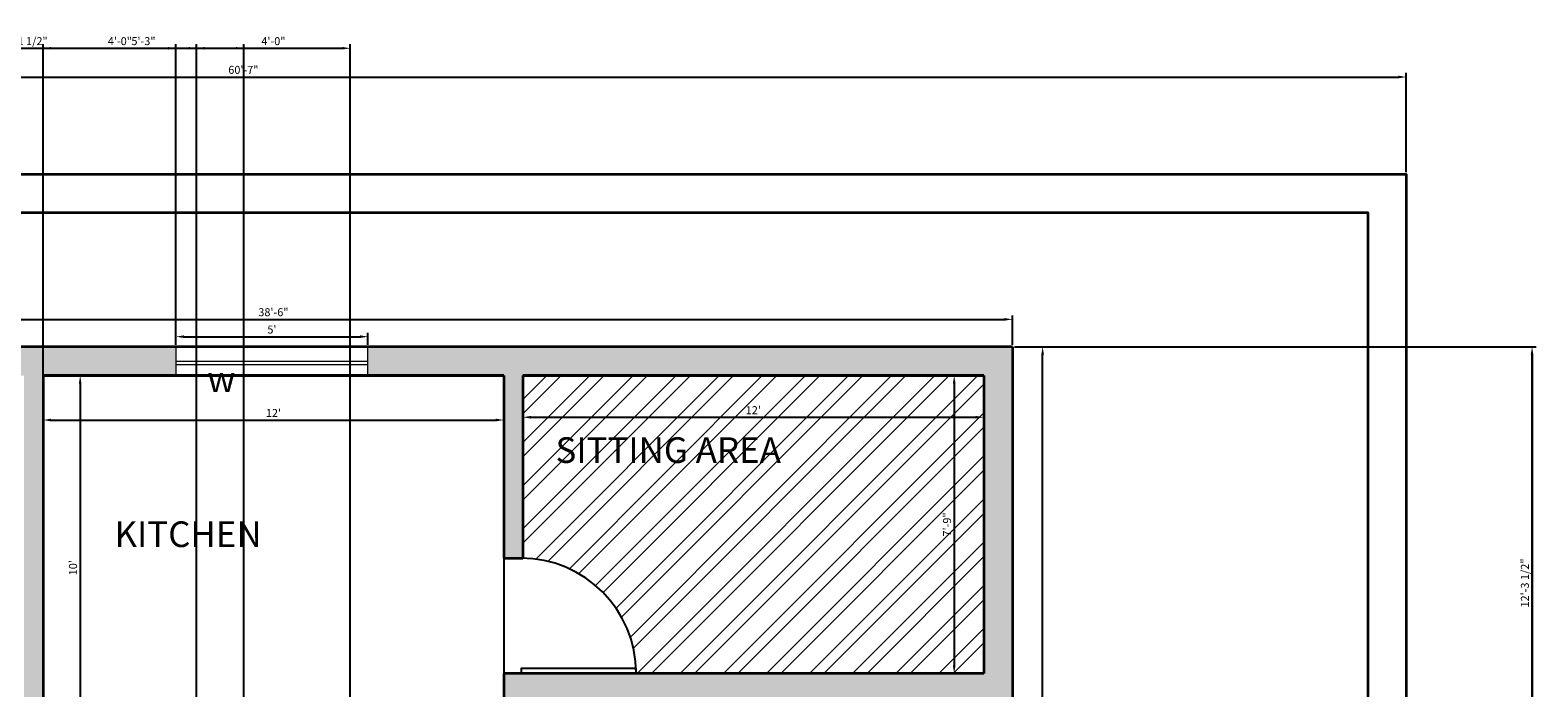
# Model space of a CAD drawing. Units: inches. Extents: x 2901 to 5923, y 918 to 2827.
# Tile 14 of 16: x 4585 to 5056, y 1524 to 1729. Entities that reach past the tile are written whole.
import ezdxf

# ---------------------------------------------------------------- set-up
doc = ezdxf.new("R2010")
doc.units = ezdxf.units.IN
for name, color, linetype, lineweight in [('A-ANNO-DIMS', 2, 'Continuous', 18), ('A-ANNO-TEXT', 7, 'Continuous', 18), ('A-AREA-IDEN', 7, 'Continuous', 25), ('A-FLOR-PATT', 252, 'Continuous', 13), ('A-GLAZ', 4, 'Continuous', 18), ('A-WALL-PATT', 7, 'Continuous', 13), ('C-PROP', 7, 'Continuous', 35), ('doors', 240, 'Continuous', 25), ('walls', 7, 'Continuous', 35)]:
    doc.layers.add(name, color=color, linetype=linetype, lineweight=lineweight)
doc.styles.get("Standard").update_dxf_attribs({"font": 'arial.ttf'})
doc.dimstyles.new('Copy of ISO-25', dxfattribs={"dimtxt": 2.5, "dimasz": 2.5, "dimexe": 1.25, "dimexo": 0.625, "dimtad": 1, "dimdec": 1, "dimlunit": 4, "dimtxsty": 'Standard', "dimcen": 2.5, "dimadec": 0, "dimazin": 0, "dimtfac": 1, "dimtdec": 1, "dimtmove": 0, "dimatfit": 3, "dimfxl": 1, "dimarcsym": 0})

# ---------------------------------------------------------------- blocks, each defined once
blk = doc.blocks.new('*U3')
for p, q in [((0, 0), (0, 6)), ((40, 0), (40, 6))]:
    blk.add_line(p, q)
blk.add_lwpolyline([(0, 0), (0, -40), (1.75, -40), (1.75, 0)], close=True)
blk.add_arc((0, 0), 40, 270, 0)
blk = doc.blocks.new('*D25')
at = {"layer": 'A-ANNO-DIMS', "color": 0, "lineweight": -2, "transparency": 16777216}
for p, q in [((4288.18, 1684.92), (4288.18, 1715.87)), ((5015.18, 1684.92), (5015.18, 1715.87)), ((4290.68, 1714.62), (5012.68, 1714.62))]:
    blk.add_line(p, q, dxfattribs=at)
at = {"layer": 'A-ANNO-DIMS', "color": 0, "transparency": 16777216}
for points in [[(4290.68, 1715.04), (4290.68, 1714.2), (4288.18, 1714.62)], [(5012.68, 1715.04), (5012.68, 1714.2), (5015.18, 1714.62)]]:
    blk.add_solid(points, dxfattribs=at)
at = {"layer": 'Defpoints', "color": 0, "transparency": 16777216}
for p in [(5015.18, 1714.62), (4288.18, 1684.29), (5015.18, 1684.29)]:
    blk.add_point(p, dxfattribs=at)
at = {"layer": 'A-ANNO-DIMS', "color": 0, "transparency": 16777216, "insert": (4651.68, 1716.52), "char_height": 2.5, "attachment_point": 5}
blk.add_mtext('60\'-7"', dxfattribs=at)
blk = doc.blocks.new('*D35')
at = {"layer": 'A-ANNO-DIMS', "color": 0, "lineweight": -2, "transparency": 16777216}
for p, q in [((4892.69, 1630.4), (4902.74, 1630.4)), ((4901.49, 1250.9), (4901.49, 1627.9)), ((4892.69, 1248.4), (4902.74, 1248.4))]:
    blk.add_line(p, q, dxfattribs=at)
at = {"layer": 'A-ANNO-DIMS', "color": 0, "transparency": 16777216}
for points in [[(4901.07, 1627.9), (4901.91, 1627.9), (4901.49, 1630.4)], [(4901.07, 1250.9), (4901.91, 1250.9), (4901.49, 1248.4)]]:
    blk.add_solid(points, dxfattribs=at)
at = {"layer": 'Defpoints', "color": 0, "transparency": 16777216}
for p in [(4892.07, 1630.4), (4901.49, 1630.4), (4892.07, 1248.4)]:
    blk.add_point(p, dxfattribs=at)
at = {"layer": 'A-ANNO-DIMS', "color": 0, "transparency": 16777216, "insert": (4899.59, 1439.4), "char_height": 2.5, "attachment_point": 5, "rotation": 90}
blk.add_mtext('31\'-10"', dxfattribs=at)
blk = doc.blocks.new('*D36')
at = {"layer": 'A-ANNO-DIMS', "color": 0, "lineweight": -2, "transparency": 16777216}
for p, q in [((4430.07, 1631.02), (4430.07, 1640.2)), ((4892.07, 1631.02), (4892.07, 1640.2)), ((4432.57, 1638.95), (4889.57, 1638.95))]:
    blk.add_line(p, q, dxfattribs=at)
at = {"layer": 'A-ANNO-DIMS', "color": 0, "transparency": 16777216}
for points in [[(4432.57, 1639.37), (4432.57, 1638.53), (4430.07, 1638.95)], [(4889.57, 1639.37), (4889.57, 1638.53), (4892.07, 1638.95)]]:
    blk.add_solid(points, dxfattribs=at)
at = {"layer": 'Defpoints', "color": 0, "transparency": 16777216}
for p in [(4892.07, 1638.95), (4430.07, 1630.4), (4892.07, 1630.4)]:
    blk.add_point(p, dxfattribs=at)
at = {"layer": 'A-ANNO-DIMS', "color": 0, "transparency": 16777216, "insert": (4661.07, 1640.85), "char_height": 2.5, "attachment_point": 5}
blk.add_mtext('38\'-6"', dxfattribs=at)
blk = doc.blocks.new('*D37')
at = {"layer": 'A-ANNO-DIMS', "color": 0, "lineweight": -2, "transparency": 16777216}
for p, q in [((4589.07, 1620.77), (4589.07, 1606.26)), ((4733.07, 1620.77), (4733.07, 1606.26)), ((4591.57, 1607.51), (4730.57, 1607.51))]:
    blk.add_line(p, q, dxfattribs=at)
at = {"layer": 'A-ANNO-DIMS', "color": 0, "transparency": 16777216}
for points in [[(4591.57, 1607.93), (4591.57, 1607.09), (4589.07, 1607.51)], [(4730.57, 1607.93), (4730.57, 1607.09), (4733.07, 1607.51)]]:
    blk.add_solid(points, dxfattribs=at)
at = {"layer": 'Defpoints', "color": 0, "transparency": 16777216}
for p in [(4589.07, 1621.4), (4733.07, 1621.4), (4733.07, 1607.51)]:
    blk.add_point(p, dxfattribs=at)
at = {"layer": 'A-ANNO-DIMS', "color": 0, "transparency": 16777216, "insert": (4661.07, 1609.39), "char_height": 2.5, "attachment_point": 5}
blk.add_mtext("12'", dxfattribs=at)
blk = doc.blocks.new('*D38')
at = {"layer": 'A-ANNO-DIMS', "color": 0, "lineweight": -2, "transparency": 16777216}
for p, q in [((4589.69, 1621.4), (4601.92, 1621.4)), ((4600.67, 1618.9), (4600.67, 1503.9)), ((4589.69, 1501.4), (4601.92, 1501.4))]:
    blk.add_line(p, q, dxfattribs=at)
at = {"layer": 'A-ANNO-DIMS', "color": 0, "transparency": 16777216}
for points in [[(4600.25, 1618.9), (4601.08, 1618.9), (4600.67, 1621.4)], [(4600.25, 1503.9), (4601.08, 1503.9), (4600.67, 1501.4)]]:
    blk.add_solid(points, dxfattribs=at)
at = {"layer": 'Defpoints', "color": 0, "transparency": 16777216}
for p in [(4589.07, 1621.4), (4589.07, 1501.4), (4600.67, 1501.4)]:
    blk.add_point(p, dxfattribs=at)
at = {"layer": 'A-ANNO-DIMS', "color": 0, "transparency": 16777216, "insert": (4598.76, 1561.4), "char_height": 2.5, "attachment_point": 5, "rotation": 90}
blk.add_mtext("10'", dxfattribs=at)
blk = doc.blocks.new('*D48')
at = {"layer": 'A-ANNO-DIMS', "color": 0, "lineweight": -2, "transparency": 16777216}
for p, q in [((4882.44, 1621.4), (4872.61, 1621.4)), ((4873.86, 1618.9), (4873.86, 1530.9)), ((4882.44, 1528.4), (4872.61, 1528.4))]:
    blk.add_line(p, q, dxfattribs=at)
at = {"layer": 'A-ANNO-DIMS', "color": 0, "transparency": 16777216}
for points in [[(4873.44, 1618.9), (4874.27, 1618.9), (4873.86, 1621.4)], [(4873.44, 1530.9), (4874.27, 1530.9), (4873.86, 1528.4)]]:
    blk.add_solid(points, dxfattribs=at)
at = {"layer": 'Defpoints', "color": 0, "transparency": 16777216}
for p in [(4883.07, 1621.4), (4873.86, 1528.4), (4883.07, 1528.4)]:
    blk.add_point(p, dxfattribs=at)
at = {"layer": 'A-ANNO-DIMS', "color": 0, "transparency": 16777216, "insert": (4871.95, 1574.9), "char_height": 2.5, "attachment_point": 5, "rotation": 90}
blk.add_mtext('7\'-9"', dxfattribs=at)
blk = doc.blocks.new('*D49')
at = {"layer": 'A-ANNO-DIMS', "color": 0, "lineweight": -2, "transparency": 16777216}
for p, q in [((4739.07, 1620.77), (4739.07, 1607.13)), ((4883.07, 1620.77), (4883.07, 1607.13)), ((4741.57, 1608.38), (4880.57, 1608.38))]:
    blk.add_line(p, q, dxfattribs=at)
at = {"layer": 'A-ANNO-DIMS', "color": 0, "transparency": 16777216}
for points in [[(4741.57, 1608.8), (4741.57, 1607.96), (4739.07, 1608.38)], [(4880.57, 1608.8), (4880.57, 1607.96), (4883.07, 1608.38)]]:
    blk.add_solid(points, dxfattribs=at)
at = {"layer": 'Defpoints', "color": 0, "transparency": 16777216}
for p in [(4739.07, 1621.4), (4883.07, 1621.4), (4883.07, 1608.38)]:
    blk.add_point(p, dxfattribs=at)
at = {"layer": 'A-ANNO-DIMS', "color": 0, "transparency": 16777216, "insert": (4811.07, 1610.26), "char_height": 2.5, "attachment_point": 5}
blk.add_mtext("12'", dxfattribs=at)
blk = doc.blocks.new('*D66')
at = {"layer": 'A-ANNO-DIMS', "color": 0, "lineweight": -2, "transparency": 16777216}
for p, q in [((4630.61, 1631.02), (4630.61, 1634.79)), ((4633.11, 1633.54), (4688.11, 1633.54)), ((4690.61, 1631.02), (4690.61, 1634.79))]:
    blk.add_line(p, q, dxfattribs=at)
at = {"layer": 'A-ANNO-DIMS', "color": 0, "transparency": 16777216}
for points in [[(4633.11, 1633.96), (4633.11, 1633.12), (4630.61, 1633.54)], [(4688.11, 1633.96), (4688.11, 1633.12), (4690.61, 1633.54)]]:
    blk.add_solid(points, dxfattribs=at)
at = {"layer": 'Defpoints', "color": 0, "transparency": 16777216}
for p in [(4690.61, 1633.54), (4630.61, 1630.4), (4690.61, 1630.4)]:
    blk.add_point(p, dxfattribs=at)
at = {"layer": 'A-ANNO-DIMS', "color": 0, "transparency": 16777216, "insert": (4660.61, 1635.43), "char_height": 2.5, "attachment_point": 5}
blk.add_mtext("5'", dxfattribs=at)
blk = doc.blocks.new('WIN-60')
for p, q in [((60, 9), (0, 9)), ((0, 9), (0, 0)), ((60, 0), (60, 9)), ((0, 4.5), (60, 4.5)), ((0, 3.5), (60, 3.5))]:
    blk.add_line(p, q)
blk = doc.blocks.new('*D89')
at = {"layer": 'A-ANNO-DIMS', "color": 0, "lineweight": -2, "transparency": 16777216}
for p, q in [((4892.69, 1630.4), (5055.73, 1630.4)), ((5054.48, 989.9), (5054.48, 1627.9)), ((4709.69, 987.4), (5055.73, 987.4))]:
    blk.add_line(p, q, dxfattribs=at)
at = {"layer": 'A-ANNO-DIMS', "color": 0, "transparency": 16777216}
for points in [[(5054.06, 1627.9), (5054.9, 1627.9), (5054.48, 1630.4)], [(5054.06, 989.9), (5054.9, 989.9), (5054.48, 987.4)]]:
    blk.add_solid(points, dxfattribs=at)
at = {"layer": 'Defpoints', "color": 0, "transparency": 16777216}
for p in [(4892.07, 1630.4), (5054.48, 1630.4), (4709.07, 987.4)]:
    blk.add_point(p, dxfattribs=at)
at = {"layer": 'A-ANNO-DIMS', "color": 0, "transparency": 16777216, "insert": (5052.58, 1308.9), "char_height": 2.5, "attachment_point": 5, "rotation": 90}
blk.add_mtext('53\'-7"', dxfattribs=at)
blk = doc.blocks.new('*D93')
at = {"layer": 'A-ANNO-DIMS', "color": 0, "lineweight": -2, "transparency": 16777216}
for p, q in [((4535.07, 1631.02), (4535.07, 1724.84)), ((4630.61, 1631.02), (4630.61, 1724.84)), ((4537.57, 1723.59), (4628.11, 1723.59))]:
    blk.add_line(p, q, dxfattribs=at)
at = {"layer": 'A-ANNO-DIMS', "color": 0, "transparency": 16777216}
for points in [[(4537.57, 1724.01), (4537.57, 1723.18), (4535.07, 1723.59)], [(4628.11, 1724.01), (4628.11, 1723.18), (4630.61, 1723.59)]]:
    blk.add_solid(points, dxfattribs=at)
at = {"layer": 'Defpoints', "color": 0, "transparency": 16777216}
for p in [(4630.61, 1723.59), (4535.07, 1630.4), (4630.61, 1630.4)]:
    blk.add_point(p, dxfattribs=at)
at = {"layer": 'A-ANNO-DIMS', "color": 0, "transparency": 16777216, "insert": (4582.84, 1725.51), "char_height": 2.5, "attachment_point": 5}
blk.add_mtext('7\'-11 1/2"', dxfattribs=at)
blk = doc.blocks.new('*D96')
at = {"layer": 'A-ANNO-DIMS', "color": 0, "lineweight": -2, "transparency": 16777216}
for p, q in [((4892.69, 1630.4), (5055.73, 1630.4)), ((5054.48, 1627.9), (5054.48, 1485.37)), ((4892.69, 1482.87), (5055.73, 1482.87))]:
    blk.add_line(p, q, dxfattribs=at)
at = {"layer": 'A-ANNO-DIMS', "color": 0, "transparency": 16777216}
for points in [[(5054.06, 1627.9), (5054.9, 1627.9), (5054.48, 1630.4)], [(5054.06, 1485.37), (5054.9, 1485.37), (5054.48, 1482.87)]]:
    blk.add_solid(points, dxfattribs=at)
at = {"layer": 'Defpoints', "color": 0, "transparency": 16777216}
for p in [(4892.07, 1630.4), (4892.07, 1482.87), (5054.48, 1482.87)]:
    blk.add_point(p, dxfattribs=at)
at = {"layer": 'A-ANNO-DIMS', "color": 0, "transparency": 16777216, "insert": (5052.56, 1556.63), "char_height": 2.5, "attachment_point": 5, "rotation": 90}
blk.add_mtext('12\'-3 1/2"', dxfattribs=at)
blk = doc.blocks.new('*D101')
at = {"layer": 'A-ANNO-DIMS', "color": 0, "lineweight": -2, "transparency": 16777216}
for p, q in [((4637.07, 1502.02), (4637.07, 1724.84)), ((4685.07, 1502.02), (4685.07, 1724.84)), ((4639.57, 1723.59), (4682.57, 1723.59))]:
    blk.add_line(p, q, dxfattribs=at)
at = {"layer": 'A-ANNO-DIMS', "color": 0, "transparency": 16777216}
for points in [[(4639.57, 1724.01), (4639.57, 1723.18), (4637.07, 1723.59)], [(4682.57, 1724.01), (4682.57, 1723.18), (4685.07, 1723.59)]]:
    blk.add_solid(points, dxfattribs=at)
at = {"layer": 'Defpoints', "color": 0, "transparency": 16777216}
for p in [(4685.07, 1723.59), (4637.07, 1501.4), (4685.07, 1501.4)]:
    blk.add_point(p, dxfattribs=at)
at = {"layer": 'A-ANNO-DIMS', "color": 0, "transparency": 16777216, "insert": (4661.07, 1725.49), "char_height": 2.5, "attachment_point": 5}
blk.add_mtext('4\'-0"', dxfattribs=at)
blk = doc.blocks.new('*D102')
at = {"layer": 'A-ANNO-DIMS', "color": 0, "lineweight": -2, "transparency": 16777216}
for p, q in [((4589.07, 1502.02), (4589.07, 1724.84)), ((4637.07, 1502.02), (4637.07, 1724.84)), ((4591.57, 1723.59), (4634.57, 1723.59))]:
    blk.add_line(p, q, dxfattribs=at)
at = {"layer": 'A-ANNO-DIMS', "color": 0, "transparency": 16777216}
for points in [[(4591.57, 1724.01), (4591.57, 1723.18), (4589.07, 1723.59)], [(4634.57, 1724.01), (4634.57, 1723.18), (4637.07, 1723.59)]]:
    blk.add_solid(points, dxfattribs=at)
at = {"layer": 'Defpoints', "color": 0, "transparency": 16777216}
for p in [(4637.07, 1723.59), (4589.07, 1501.4), (4637.07, 1501.4)]:
    blk.add_point(p, dxfattribs=at)
at = {"layer": 'A-ANNO-DIMS', "color": 0, "transparency": 16777216, "insert": (4613.07, 1725.49), "char_height": 2.5, "attachment_point": 5}
blk.add_mtext('4\'-0"', dxfattribs=at)
blk = doc.blocks.new('*D105')
at = {"layer": 'A-ANNO-DIMS', "color": 0, "lineweight": -2, "transparency": 16777216}
for p, q in [((4589.07, 1298.02), (4589.07, 1724.84)), ((4651.83, 1240.37), (4651.83, 1724.84)), ((4591.57, 1723.59), (4649.33, 1723.59))]:
    blk.add_line(p, q, dxfattribs=at)
at = {"layer": 'A-ANNO-DIMS', "color": 0, "transparency": 16777216}
for points in [[(4591.57, 1724.01), (4591.57, 1723.18), (4589.07, 1723.59)], [(4649.33, 1724.01), (4649.33, 1723.18), (4651.83, 1723.59)]]:
    blk.add_solid(points, dxfattribs=at)
at = {"layer": 'Defpoints', "color": 0, "transparency": 16777216}
for p in [(4651.83, 1723.59), (4589.07, 1297.4), (4651.83, 1239.74)]:
    blk.add_point(p, dxfattribs=at)
at = {"layer": 'A-ANNO-DIMS', "color": 0, "transparency": 16777216, "insert": (4620.45, 1725.5), "char_height": 2.5, "attachment_point": 5}
blk.add_mtext('5\'-3"', dxfattribs=at)

msp = doc.modelspace()

# ---------------------------------------------------------------- hatches: boundary and pattern name
at = {"layer": 'A-FLOR-PATT'}
h = msp.add_hatch(dxfattribs=at)
h.set_pattern_fill('ANSI32', color=256)
h.paths.add_polyline_path([(4883.07, 1621.4), (4739.07, 1621.4), (4739.07, 1564.39, -0.396616), (4774.43, 1529.97), (4774.46, 1529.97), (4774.46, 1528.4), (4883.07, 1528.4)])
h.paths.add_polyline_path([(4733.07, 1143.4), (4685.07, 1143.4), (4685.07, 1147.03), (4684.01, 1147.03), (4684.01, 1171.22, 0.413071), (4660.87, 1146.06, 0.412532), (4638.11, 1170.77), (4638.11, 1146.97), (4637.07, 1143.4), (4589.07, 1143.4), (4589.07, 1029.4), (4733.07, 1029.4)])
h.paths.add_polyline_path([(4620.35, 1086.26, -0.333335), (4622.56, 1084.04), (4622.56, 1084.04), (4712.62, 1084.04, -0.333335), (4714.84, 1086.26), (4718.53, 1086.26, -0.376086), (4721.48, 1084.04), (4721.48, 1062.64), (4721.48, 1041.23, -0.333387), (4718.96, 1039.01), (4714.84, 1039.01, -0.333335), (4712.62, 1041.23), (4712.62, 1041.23), (4622.56, 1041.23, -0.333335), (4620.35, 1039.01), (4616.66, 1039.01, -0.376086), (4613.71, 1041.23), (4613.71, 1062.63), (4613.71, 1084.04, -0.333387), (4616.23, 1086.26)], flags=16)
h.paths.add_polyline_path([(4638.8, 1084.04), (4643.23, 1078.14), (4678.67, 1078.14), (4687.53, 1084.04), (4687.53, 1071.49), (4718.53, 1067.06), (4718.53, 1062.64), (4718.53, 1058.21), (4687.53, 1053.78), (4687.53, 1041.23), (4678.67, 1047.13), (4643.23, 1047.13), (4638.8, 1041.23), (4638.8, 1062.63)], flags=0)
at = {"layer": 'A-WALL-PATT'}
h = msp.add_hatch(color=256, dxfattribs=at)
h.dxf.hatch_style = 1
h.paths.add_polyline_path([(4439.07, 1447.4), (4583.07, 1447.4), (4583.07, 1340.4), (4589.07, 1340.4), (4589.07, 1453.4), (4589.07, 1455.39), (4583.07, 1455.39), (4583.07, 1453.4), (4439.07, 1453.4), (4439.07, 1501.84), (4430.07, 1501.84), (4430.07, 1399.4), (4439.07, 1399.4)])
h.paths.add_polyline_path([(4439.07, 1621.4), (4487.07, 1621.4), (4487.07, 1630.4), (4430.07, 1630.4), (4430.07, 1561.84), (4439.07, 1561.84)])
h.paths.add_polyline_path([(4630.61, 1630.4), (4535.07, 1630.4), (4535.07, 1621.4), (4583.07, 1621.4), (4583.07, 1495.4), (4589.07, 1495.4), (4637.07, 1495.4), (4637.07, 1501.4), (4589.07, 1501.4), (4589.07, 1621.4), (4630.61, 1621.4)])
h.paths.add_polyline_path([(4892.07, 1630.4), (4690.61, 1630.4), (4690.61, 1621.4), (4733.07, 1621.4), (4733.07, 1564.4), (4739.07, 1564.4), (4739.07, 1621.4), (4883.07, 1621.4), (4883.07, 1528.4), (4739.07, 1528.4), (4733.07, 1528.4), (4733.07, 1501.4), (4685.07, 1501.4), (4685.07, 1495.4), (4739.07, 1495.4), (4739.07, 1519.4), (4787.07, 1519.4), (4787.07, 1423.4), (4739.07, 1423.4), (4739.07, 1456.67), (4733.07, 1456.67), (4733.07, 1340.4), (4739.07, 1340.4), (4739.07, 1417.4), (4787.07, 1417.4), (4793.07, 1417.4), (4793.07, 1423.4), (4793.07, 1519.4), (4883.07, 1519.4), (4883.07, 1482.87), (4892.07, 1482.87)])
h.paths.add_polyline_path([(4892.07, 1458.87), (4883.07, 1458.87), (4883.07, 1423.4), (4823.07, 1423.4), (4823.07, 1417.4), (4883.07, 1417.4), (4883.07, 1363.31), (4892.07, 1363.31)], flags=17)
h.paths.add_polyline_path([(4892.07, 1303.31), (4883.07, 1303.31), (4883.07, 1255.4), (4739.07, 1255.4), (4739.07, 1304.4), (4733.07, 1304.4), (4733.07, 1303.4), (4733.07, 1297.4), (4733.07, 1255.4), (4733.07, 1248.4), (4811.07, 1248.4), (4811.07, 1212.16), (4820.07, 1212.16), (4820.07, 1248.4), (4892.07, 1248.4)])
h.paths.add_polyline_path([(4820.07, 1182.16), (4811.07, 1182.16), (4811.07, 1152.4), (4685.07, 1152.4), (4685.07, 1147.03), (4685.07, 1143.4), (4733.07, 1143.4), (4811.07, 1143.4), (4814.07, 1143.4), (4820.07, 1143.4)])
h.paths.add_polyline_path([(4637.07, 1152.4), (4589.07, 1152.4), (4589.07, 1153.4), (4583.86, 1153.4), (4583.07, 1153.4), (4583.07, 1152.4), (4511.07, 1152.4), (4511.07, 1182.16), (4502.07, 1182.16), (4502.07, 1143.4), (4568.07, 1143.4), (4583.07, 1143.4), (4583.07, 1023.4), (4739.07, 1023.4), (4739.07, 1143.4), (4733.07, 1143.4), (4733.07, 1029.4), (4589.07, 1029.4), (4589.07, 1143.4), (4637.07, 1143.4), (4637.07, 1146.97)])
h.paths.add_polyline_path([(4511.07, 1246.4), (4583.07, 1246.4), (4583.07, 1188.4), (4589.07, 1188.4), (4589.07, 1246.4), (4589.07, 1248.4), (4589.07, 1255.4), (4589.07, 1297.4), (4697.07, 1297.4), (4697.07, 1303.4), (4589.07, 1303.4), (4589.07, 1304.4), (4583.07, 1304.4), (4583.07, 1255.4), (4439.07, 1255.4), (4439.07, 1261.4), (4439.07, 1351.4), (4430.07, 1351.4), (4430.07, 1252.4), (4430.07, 1246.4), (4439.07, 1246.4), (4487.07, 1246.4), (4502.07, 1246.4), (4502.07, 1212.16), (4511.07, 1212.16)])

# ---------------------------------------------------------------- linework, layer by layer
at = {"layer": 'C-PROP'}
msp.add_lwpolyline([(4288.18, 1684.29), (5015.18, 1684.29), (5015.18, 958.29), (4288.18, 958.29)], close=True, dxfattribs=at)
msp.add_lwpolyline([(5003.18, 978.26), (5003.18, 970.29), (4300.18, 970.29), (4300.18, 1672.29), (5003.18, 1672.29), (5003.18, 1132.27)], dxfattribs=at)
at = {"layer": 'doors'}
msp.add_line((4733.07, 1564.39), (4733.07, 1528.4), dxfattribs=at)
at = {"layer": 'walls'}
for p, q in [((4892.07, 1630.4), (4892.07, 1248.4)), ((4589.07, 1621.4), (4589.07, 1501.4)), ((4589.07, 1621.4), (4733.07, 1621.4)), ((4733.07, 1621.4), (4690.61, 1621.4)), ((4733.07, 1621.4), (4733.07, 1564.4)), ((4739.07, 1621.4), (4739.07, 1564.4)), ((4739.07, 1621.4), (4883.07, 1621.4)), ((4883.07, 1621.4), (4883.07, 1528.4)), ((4733.07, 1564.4), (4739.07, 1564.4)), ((4739.07, 1528.4), (4733.07, 1528.4)), ((4733.07, 1528.4), (4733.07, 1501.4)), ((4883.07, 1528.4), (4739.07, 1528.4))]:
    msp.add_line(p, q, dxfattribs=at)
for points in [[(4892.07, 1630.4), (4430.07, 1630.4), (4430.07, 1252.4)], [(4733.07, 1621.4), (4589.07, 1621.4)], [(4883.07, 1621.4), (4739.07, 1621.4)]]:
    msp.add_lwpolyline(points, dxfattribs=at)

# ---------------------------------------------------------------- block references
at = {"layer": 'A-GLAZ'}
msp.add_blockref('WIN-60', (4630.6, 1621.4), dxfattribs=at)
at = {"layer": 'doors', "xscale": 0.8998794252002142, "yscale": 0.8998794252002142, "zscale": 0.8998794252002142, "rotation": 90}
msp.add_blockref('*U3', (4738.47, 1528.4), dxfattribs=at)

# ---------------------------------------------------------------- texts
at = {"layer": 'A-ANNO-TEXT'}
msp.add_text('w', height=8, dxfattribs=at).set_placement((4640.42, 1616.28))
at = {"layer": 'A-AREA-IDEN'}
for s, p in [('SITTING AREA', (4749.24, 1594.12)), ('KITCHEN', (4611.38, 1567.86))]:
    msp.add_text(s, height=8, dxfattribs=at).set_placement(p)

# ---------------------------------------------------------------- dimensions: what is measured, and where the dimension line sits
at = {"layer": 'A-ANNO-DIMS'}
for base, p1, p2, override, picture, middle in [((4630.61, 1723.59), (4535.07, 1630.4), (4630.61, 1630.4), {"dimdec": 1, "dimlfac": 1, "dimrnd": 0, "dimzin": 1, "dimdsep": 46, "dimlunit": 4, "dimfrac": 2}, '*D93', (4582.84, 1725.51)), ((4637.07, 1723.59), (4589.07, 1501.4), (4637.07, 1501.4), {"dimdec": 1, "dimlfac": 1, "dimrnd": 0, "dimzin": 1, "dimdsep": 46, "dimlunit": 4, "dimfrac": 2}, '*D102', (4613.07, 1725.49)), ((4651.83, 1723.59), (4589.07, 1297.4), (4651.83, 1239.74), {"dimdec": 1, "dimlfac": 1, "dimrnd": 0, "dimzin": 1, "dimdsep": 46, "dimlunit": 4, "dimfrac": 2}, '*D105', (4620.45, 1725.5)), ((4685.07, 1723.59), (4637.07, 1501.4), (4685.07, 1501.4), {"dimdec": 1, "dimlfac": 1, "dimrnd": 0, "dimzin": 1, "dimdsep": 46, "dimlunit": 4, "dimfrac": 2}, '*D101', (4661.07, 1725.49)), ((5015.18, 1714.62), (4288.18, 1684.29), (5015.18, 1684.29), {"dimclrd": 0, "dimclre": 0, "dimclrt": 0}, '*D25', (4651.68, 1716.52)), ((4892.07, 1638.95), (4430.07, 1630.4), (4892.07, 1630.4), {"dimclrd": 0, "dimclre": 0, "dimclrt": 0}, '*D36', (4661.07, 1640.85)), ((4690.61, 1633.54), (4630.61, 1630.4), (4690.61, 1630.4), {"dimclrd": 0, "dimclre": 0, "dimclrt": 0}, '*D66', (4660.61, 1635.43)), ((4733.07, 1607.51), (4589.07, 1621.4), (4733.07, 1621.4), {"dimclrd": 0, "dimclre": 0, "dimclrt": 0}, '*D37', (4661.07, 1609.39)), ((4883.07, 1608.38), (4739.07, 1621.4), (4883.07, 1621.4), {"dimclrd": 0, "dimclre": 0, "dimclrt": 0}, '*D49', (4811.07, 1610.26))]:
    dim = msp.add_linear_dim(base=base, p1=p1, p2=p2, dimstyle='Copy of ISO-25', override=override, dxfattribs=at)
    dim.commit()
    dim.dimension.update_dxf_attribs({"geometry": picture, "text_midpoint": middle})
for base, p1, p2, override, picture, middle in [((5054.48, 1630.4), (4709.07, 987.4), (4892.07, 1630.4), {"dimdec": 1, "dimlfac": 1, "dimrnd": 0, "dimzin": 1, "dimdsep": 46, "dimlunit": 4, "dimfrac": 2}, '*D89', (5052.58, 1308.9)), ((4901.49, 1630.4), (4892.07, 1248.4), (4892.07, 1630.4), {"dimclrd": 0, "dimclre": 0, "dimclrt": 0}, '*D35', (4899.59, 1439.4)), ((5054.48, 1482.87), (4892.07, 1630.4), (4892.07, 1482.87), {"dimdec": 1, "dimlfac": 1, "dimrnd": 0, "dimzin": 1, "dimdsep": 46, "dimlunit": 4, "dimfrac": 2}, '*D96', (5052.56, 1556.63)), ((4600.67, 1501.4), (4589.07, 1621.4), (4589.07, 1501.4), {"dimclrd": 0, "dimclre": 0, "dimclrt": 0}, '*D38', (4598.76, 1561.4)), ((4873.86, 1528.4), (4883.07, 1621.4), (4883.07, 1528.4), {"dimclrd": 0, "dimclre": 0, "dimclrt": 0}, '*D48', (4871.95, 1574.9))]:
    dim = msp.add_linear_dim(base=base, p1=p1, p2=p2, angle=90, dimstyle='Copy of ISO-25', override=override, dxfattribs=at)
    dim.commit()
    dim.dimension.update_dxf_attribs({"geometry": picture, "text_midpoint": middle})

doc.saveas('drawing.dxf')
